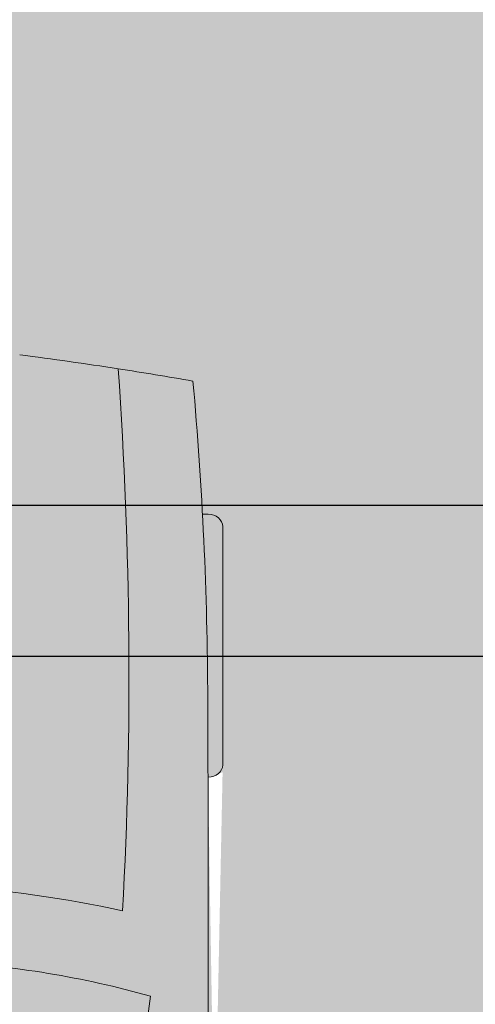
# Model space of a CAD drawing. Units: inches. Extents: x 389 to 971, y 148 to 870.
# Tile 2 of 14: x 529 to 565, y 349 to 428. Entities that reach past the tile are written whole.
import ezdxf

# ---------------------------------------------------------------- set-up
doc = ezdxf.new("R2010")
doc.units = ezdxf.units.IN
doc.header["$MEASUREMENT"] = 0
for name, color, linetype, lineweight in [('A-ANNO-DIMS', 2, 'Continuous', 18), ('C-VEHI', 8, 'Continuous', 13), ('L-GRND-BASE-PATT', 8, 'Continuous', 13)]:
    doc.layers.add(name, color=color, linetype=linetype, lineweight=lineweight)
doc.layers.add('C-VEHI-PATT', color=18, linetype='Continuous', lineweight=13, true_color=0x000000)
doc.layers.add('L-GRND-PATT', color=39, linetype='Continuous', lineweight=13, true_color=0x603913)
doc.styles.get("Standard").update_dxf_attribs({"font": 'arial.ttf'})
doc.dimstyles.get("Standard").update_dxf_attribs({"dimtxt": 8, "dimasz": 8, "dimexe": 0.18, "dimexo": 0.0625, "dimgap": 0.09, "dimtad": 0, "dimtih": 1, "dimtoh": 1, "dimdec": 0, "dimzin": 0, "dimdsep": 46, "dimlunit": 3, "dimtxsty": 'Standard', "dimcen": 0.09, "dimadec": 0, "dimazin": 0, "dimtfac": 1, "dimtdec": 0, "dimtofl": 0, "dimtmove": 0, "dimatfit": 3, "dimfxl": 1, "dimtolj": 1, "dimtzin": 0, "dimarcsym": 0})

# ---------------------------------------------------------------- blocks, each defined once
blk = doc.blocks.new('*U7')
for p, q in [((46.55368679439944, 38.88847654282876), (22.35054758993934, 38.88847654282876)), ((21.10406751471477, 37.40863046792069), (21.10406751471477, 36.83230215753705)), ((47.80016686962392, 37.39011648242055), (47.80016686962392, 37.40863046792069)), ((70.0302824853563, 31.53613089391356), (86.40615155322342, 29.35124891408057))]:
    blk.add_line(p, q)
for centre, major_axis, ratio, start_param, end_param in [((22.35054758993934, 37.40863046792072), (2.08e-14, -1.479846074908118), 0.842303869543976, 3.141592653589776, 4.712388980384677), ((46.55368679439944, 37.40863046792072), (2.2e-14, 1.479846074908118), 0.8423038695439758, -1.570796326794884, 1.73e-14), ((41.19115208863305, -490.8631038926156), (1.294e-13, 528.2339998381949), 0.8423038695439741, 0.0028100083536837, 0.0755983031096952), ((64.48199294511879, -10555.61767587835), (1.907644e-10, 10593.02630634627), 0.842303869543847, -0.0133969486112073, 0.0027970409639888), ((266.0300214172791, -27.52442688366631), (1.966072e-10, 313.3077612809058), 0.8423038695435284, 1.367075990158062, 1.391760499156098), ((135.2911776514449, 5.387441675478555), (2.2715e-12, 81.77258453065997), 0.8423038695439563, 1.245306111696802, 1.507880129813836), ((37.47375371777758, -593.9621830607928), (6.21e-14, -623.32820996736), 0.8423038695439826, 3.09604606856106, 3.200911180495224), ((259.1750197310735, -27.52442688366614), (1.506617e-10, -305.3028914627677), 0.8423038695443789, 4.528606069860317, 4.561837674556238), ((134.4003789125686, 5.387441675477674), (4.276e-13, -89.7774543484738), 0.84230386954398, 4.44948196380473, 4.652344057257214)]:
    blk.add_ellipse(centre, major_axis=major_axis, ratio=ratio, start_param=start_param, end_param=end_param)
blk = doc.blocks.new('*D53')
at = {"layer": 'A-ANNO-DIMS', "color": 0, "lineweight": -2, "transparency": 16777216}
for p, q in [((397.8910240000004, 396.9189020000002), (397.8910240000004, 404.9189020000001)), ((690.1535240000002, 388.9189020000003), (397.7110240000004, 388.9189020000002)), ((690.1535240000002, 376.9189020000001), (397.7110240000005, 376.9189020000001)), ((397.8910240000005, 368.9189020000001), (397.8910240000005, 360.918902))]:
    blk.add_line(p, q, dxfattribs=at)
at = {"layer": 'A-ANNO-DIMS', "color": 0, "transparency": 16777216}
for points in [[(396.5576906666671, 396.9189020000002), (399.2243573333337, 396.9189020000002), (397.8910240000004, 388.9189020000002)], [(396.5576906666671, 368.9189020000001), (399.2243573333338, 368.9189020000001), (397.8910240000005, 376.9189020000001)]]:
    blk.add_solid(points, dxfattribs=at)
at = {"layer": 'Defpoints', "color": 0, "transparency": 16777216}
for p in [(397.8910240000004, 388.9189020000002), (690.2160240000001, 388.9189020000003), (690.2160240000001, 376.9189020000001)]:
    blk.add_point(p, dxfattribs=at)
at = {"layer": 'A-ANNO-DIMS', "color": 0, "transparency": 16777216, "insert": (397.8910240000004, 382.9189019999999), "char_height": 8, "attachment_point": 5}
blk.add_mtext('\\A1;12', dxfattribs=at)

msp = doc.modelspace()

# ---------------------------------------------------------------- hatches: boundary and pattern name
at = {"layer": 'C-VEHI-PATT'}
h = msp.add_hatch(color=256, dxfattribs=at)
h.dxf.hatch_style = 1
edge = h.paths.add_edge_path()
edge.add_ellipse((550.9021553826709, 381.4331108862803), major_axis=(-43.99405423656321, 1.9369e-12), ratio=0.8423038695439613, start_angle=-29.43856959797762, end_angle=1.8189894035458565e-12, ccw=False)
edge.add_line((514.3535105156315, 402.059641051582), (514.3535105156315, 404.7525403567118))
edge.add_ellipse((514.3535105156316, 404.2643898676136), major_axis=(0.5795420236673633, 2e-16), ratio=0.8423038695437671, start_angle=90.00000000001334, end_angle=127.9331304598466)
edge.add_line((514.0354569934393, 404.6724605914631), (509.5535496243029, 402.1940957519602))
edge.add_ellipse((473.3138688667988, 564.9222417143382), major_axis=(196.5636751472093, 8.4793e-12), ratio=0.8423038695439335, start_angle=-80.7434339928015, end_angle=-77.44506735586577, ccw=False)
edge.add_ellipse((535.9119176052684, 201.7546502845751), major_axis=(239.1273775699096, 1.008988e-10), ratio=0.842303869543627, start_angle=100.2095389971183, end_angle=102.4446272934191)
edge.add_ellipse((979.5722266908713, 375.4013592680145), major_axis=(-488.2195497741742, 7.7268e-12), ratio=0.842303869543895, start_angle=-2.863714607837472, end_angle=2.198540565955285)
edge.add_ellipse((510.1338164488812, 299.4839331720496), major_axis=(70.3178640738586, 3.814e-12), ratio=0.8423038695439212, start_angle=94.08241069114638, end_angle=107.71995322274631, ccw=False)
edge.add_line((505.914122382133, 358.6062023341113), (522.79289864913, 358.606202334111))
edge.add_ellipse((518.5732045823792, 299.4839331720493), major_axis=(-70.31786407385354, 1.4408e-12), ratio=0.8423038695439844, start_angle=252.2800467772501, end_angle=265.91758930884987, ccw=False)
edge.add_ellipse((49.13479434038987, 375.4013592680261), major_axis=(-488.2195497741754, 2.5232e-12), ratio=0.8423038695439587, start_angle=177.8014594340444, end_angle=182.8637146078372)
edge.add_ellipse((492.795103425985, 201.7546502845724), major_axis=(239.12737756976, 4.82267e-11), ratio=0.8423038695441539, start_angle=77.5553727065425, end_angle=79.79046100284327)
edge.add_ellipse((555.3931521644682, 564.9222417143374), major_axis=(-196.5636751472384, 3.62381e-11), ratio=0.8423038695438114, start_angle=77.4450673558726, end_angle=80.74343399280832, ccw=False)
edge.add_line((519.1534714069603, 402.19409575196), (514.671564037824, 404.6724605914631))
edge.add_ellipse((514.3535105156316, 404.2643898676136), major_axis=(0.5795420236673633, 2e-16), ratio=0.8423038695437671, start_angle=52.06686954015338, end_angle=90.00000000001334)
edge.add_line((514.3535105156315, 404.7525403567118), (514.3535105156315, 402.0596410515821))
edge.add_ellipse((477.8048656485917, 381.4331108862812), major_axis=(-43.99405423656326, 6.67e-13), ratio=0.8423038695439753, start_angle=180.0000000000002, end_angle=209.4385695979796, ccw=False)
edge.add_line((521.7989198851549, 381.4331108862806), (521.7989198851549, 379.5923831537828))
edge.add_line((521.7989198851549, 379.5923831537828), (523.2258361412675, 379.5923831537828))
edge.add_ellipse((523.0896049791924, 379.1042326646847), major_axis=(0.5795420236669786, 3.601e-13), ratio=0.8423038695443263, start_angle=45.519789117397124, end_angle=89.99999999996442, ccw=False)
edge.add_line((523.4589887688404, 379.4803801228631), (527.8015488731598, 376.4548385069232))
edge.add_line((527.8015488731598, 376.4548385069232), (527.8015488731597, 364.8548231745798))
edge.add_ellipse((524.8002343791572, 364.9712406163019), major_axis=(0.279312372030448, 4.96584264291768), ratio=0.6038335755719146, start_angle=106.34259195429831, end_angle=270.9979857249735, ccw=False)
edge.add_line((521.7989198851548, 364.2715269884119), (521.7989198851549, 381.4331108862806))
edge.add_ellipse((477.8048656485917, 381.4331108862812), major_axis=(-43.99405423656326, 6.67e-13), ratio=0.8423038695439753, start_angle=180.0000000000001, end_angle=209.4385695979795)
edge.add_ellipse((550.9021553826709, 381.4331108862803), major_axis=(-43.99405423656321, 1.9369e-12), ratio=0.8423038695439613, start_angle=-29.43856959797755, end_angle=1.8539e-12)
edge.add_line((506.9081011461076, 381.43311088628), (506.9081011461074, 364.2715269884121))
edge.add_ellipse((503.9067866521049, 364.9712406163021), major_axis=(-0.2793123720310282, 4.965842642917721), ratio=0.6038335755718928, start_angle=89.00201427501901, end_angle=253.6574080456941, ccw=False)
edge.add_line((500.9054721581025, 364.8548231745812), (500.9054721581025, 376.4548385069235))
edge.add_line((500.9054721581025, 376.4548385069235), (505.3530060491612, 379.5535172937331))
edge.add_ellipse((505.61741605207, 379.1042326646849), major_axis=(-0.5795420236672051, 1.236e-13), ratio=0.842303869543997, start_angle=-89.99999999998778, end_angle=-45.51978911742469, ccw=False)
edge.add_line((505.61741605207, 379.5923831537831), (506.9081011461076, 379.5923831537831))
edge.add_line((506.9081011461076, 379.5923831537831), (506.9081011461076, 381.43311088628))
h = msp.add_hatch(color=256, dxfattribs=at)
h.dxf.hatch_style = 1
edge = h.paths.add_edge_path()
edge.add_ellipse((492.795103425985, 201.7546502845724), major_axis=(239.12737756976, 4.82267e-11), ratio=0.8423038695441539, start_angle=77.5553727065425, end_angle=79.79046100284327)
edge.add_ellipse((555.3931521644682, 564.9222417143374), major_axis=(-196.5636751472384, 3.62381e-11), ratio=0.8423038695438114, start_angle=77.4450673558726, end_angle=80.74343399280832, ccw=False)
edge.add_line((519.1534714069603, 402.19409575196), (519.1534714069603, 394.0892586662818))
edge.add_ellipse((477.8048656485917, 381.4331108862812), major_axis=(-43.99405423656326, 6.67e-13), ratio=0.8423038695439753, start_angle=180.0000000000002, end_angle=197.0185128172791, ccw=False)
edge.add_line((521.7989198851549, 381.4331108862806), (521.7989198851549, 379.5923831537828))
edge.add_line((521.7989198851549, 379.5923831537828), (523.1794038652976, 379.5923831537828))
edge.add_ellipse((523.0896049791924, 379.1042326646847), major_axis=(0.5795420236669786, 3.601e-13), ratio=0.8423038695443263, start_angle=45.519789117397124, end_angle=89.99999999996442, ccw=False)
edge.add_line((523.4589887688405, 379.480380122863), (527.8015488731598, 376.4548385069232))
edge.add_line((527.8015488731598, 376.4548385069232), (527.8015488731597, 364.8548231745798))
edge.add_ellipse((524.8002343791572, 364.9712406163019), major_axis=(0.279312372030448, 4.96584264291768), ratio=0.6038335755719146, start_angle=106.34259195429831, end_angle=270.9979857249735, ccw=False)
edge.add_line((521.7989198851548, 364.2715269884119), (521.7989198851549, 381.4331108862806))
edge.add_ellipse((477.8048656485917, 381.4331108862812), major_axis=(-43.99405423656326, 6.67e-13), ratio=0.8423038695439753, start_angle=180.0000000000001, end_angle=197.018512817279)
edge.add_line((519.1534714069603, 394.0892586662818), (519.1534714069603, 358.6062023341111))
edge.add_line((519.1534714069603, 358.6062023341111), (522.79289864913, 358.606202334111))
edge.add_ellipse((518.5732045823792, 299.4839331720493), major_axis=(-70.31786407385354, 1.4408e-12), ratio=0.8423038695439844, start_angle=252.2800467772501, end_angle=265.91758930884987, ccw=False)
edge.add_ellipse((49.13479434038987, 375.4013592680261), major_axis=(-488.2195497741754, 2.5232e-12), ratio=0.8423038695439587, start_angle=177.8014594340444, end_angle=182.8637146078372)
h = msp.add_hatch(color=256, dxfattribs=at)
h.dxf.hatch_style = 1
edge = h.paths.add_edge_path(flags=16)
edge.add_ellipse((3386.011413077446, 329.726312794031), major_axis=(-2896.629999631248, 1.069454e-10), ratio=0.8423038695494893, start_angle=-0.1208973690315247, end_angle=0.3640763488915013, ccw=False)
edge.add_line((489.3905023836935, 335.8383575186984), (486.2179253655185, 346.1978202249628))
edge.add_ellipse((8782.002602781096, 354.247254279773), major_axis=(-8295.790181758603, 9.87839e-10), ratio=0.8423038695486498, start_angle=0.0555943135052214, end_angle=0.3777641939157137)
edge.add_line((486.4665645878948, 299.5520931219791), (489.4638383140943, 311.3204429697198))
edge = h.paths.add_edge_path(flags=16)
edge.add_ellipse((512.1608573463288, 287.5825181681774), major_axis=(62.33048198263887, 2.0798e-12), ratio=0.8423038695439498, start_angle=94.8700695971331, end_angle=112.791914877584)
edge.add_line((491.3642517254777, 337.0752369161335), (489.6529508739416, 349.9015767089268))
edge.add_ellipse((510.1338164488795, 298.7862183048575), major_axis=(64.04807894948699, 3.9006e-12), ratio=0.8423038695439252, start_angle=94.27742096304979, end_angle=111.83495379670401, ccw=False)
edge.add_line((506.1068129054811, 352.6274231954524), (522.600208125781, 352.6274231954521))
edge.add_ellipse((518.5732045823798, 298.7862183048586), major_axis=(64.04807894948067, 3.24e-14), ratio=0.8423038695439885, start_angle=68.16504620328948, end_angle=85.72257903694378, ccw=False)
edge.add_line((539.05407015732, 349.9015767089259), (537.3427693057835, 337.0752369161327))
edge.add_ellipse((516.5461636849332, 287.5825181681899), major_axis=(62.33048198262021, 1.5954e-12), ratio=0.8423038695439995, start_angle=67.20808512240782, end_angle=85.12993040286212)
edge.add_line((521.0080028322477, 339.9490379899644), (507.6990181990146, 339.9490379899646))
edge = h.paths.add_edge_path(flags=16)
edge.add_ellipse((514.3535105156315, 391.3730654902235), major_axis=(-115.1512533244504, 1.8736e-12), ratio=0.8423038695439684, start_angle=76.4018653097696, end_angle=103.5981346902308)
edge.add_line((537.3427693057832, 296.3333211885938), (537.342769305783, 281.5897392316151))
edge.add_ellipse((514.3535105156313, 376.6294835332447), major_axis=(-115.1512533244486, 9.02e-13), ratio=0.8423038695439828, start_angle=76.40186530976922, end_angle=103.59813469023032, ccw=False)
edge.add_line((491.3642517254773, 281.5897392316156), (491.3642517254774, 296.3333211885945))
edge = h.paths.add_edge_path()
edge.add_ellipse((8782.002602781105, 354.2472542798386), major_axis=(-8296.949265805946, 5.39345e-11), ratio=0.8423038695428886, start_angle=0.3838667787920247, end_angle=0.5282714718170651)
edge.add_ellipse((8782.002602781105, 354.2472542798386), major_axis=(-8296.949265805946, 5.39345e-11), ratio=0.8423038695428886, start_angle=0.5282714718170651, end_angle=0.6465540970606384)
edge.add_ellipse((488.1158467995968, 260.6509346628684), major_axis=(2.318168094668909, 7.48e-14), ratio=0.8423038695439647, start_angle=180.6465540970884, end_angle=269.9999999999081)
edge.add_line((488.115846799593, 258.6983327064755), (491.3642517254771, 258.6983327064753))
edge.add_line((491.3642517254771, 258.6983327064753), (491.3642517254771, 274.201106836649))
edge.add_ellipse((493.6824198201462, 273.9438556676354), major_axis=(-2.318168094668919, 1.896e-13), ratio=0.8423038695439611, start_angle=-89.99999999999523, end_angle=4.718003765447065e-12, ccw=False)
edge.add_line((493.6824198201462, 275.8964576240284), (535.3300149439905, 275.8964576240277))
edge.add_ellipse((535.024601211114, 273.9438556676347), major_axis=(2.318168094668976, 2.946e-13), ratio=0.8423038695439647, start_angle=-7.275957614183426e-12, end_angle=89.99999999998943, ccw=False)
edge.add_line((537.342769305783, 273.9438556676347), (537.3427693057827, 258.698332706474))
edge.add_line((537.3427693057827, 258.698332706474), (540.591174231666, 258.6983327064739))
edge.add_ellipse((540.5911742316634, 260.6509346628669), major_axis=(-2.318168094668839, 2.143e-13), ratio=0.8423038695440144, start_angle=90.00000000008203, end_angle=179.3534459029346)
edge.add_ellipse((-7753.295581726658, 354.2472542799028), major_axis=(-8296.949265782761, 2.068448e-10), ratio=0.8423038695442414, start_angle=179.3534459029388, end_angle=179.3813568036815)
edge.add_ellipse((-7753.295581726658, 354.2472542799028), major_axis=(-8296.949265782761, 2.068448e-10), ratio=0.8423038695442414, start_angle=179.3813568036815, end_angle=179.4717285281828)
edge.add_ellipse((-7753.295581726658, 354.2472542799028), major_axis=(-8296.949265782761, 2.068448e-10), ratio=0.8423038695442414, start_angle=179.4717285281828, end_angle=179.6161332212082)
edge.add_ellipse((-7753.295581726658, 354.2472542799028), major_axis=(-8296.949265782761, 2.068448e-10), ratio=0.8423038695442414, start_angle=179.6161332212082, end_angle=180.090229088595)
edge.add_ellipse((-7753.295581726658, 354.2472542799028), major_axis=(-8296.949265782761, 2.068448e-10), ratio=0.8423038695442414, start_angle=180.090229088595, end_angle=180.134986576859)
edge.add_ellipse((129.8867725257751, 372.4897205359271), major_axis=(-413.7373561031673, 2.44623e-11), ratio=0.8423038695441432, start_angle=180.1806905311865, end_angle=182.1799503136479)
edge.add_ellipse((129.8867725257751, 372.4897205359271), major_axis=(-413.7373561031673, 2.44623e-11), ratio=0.8423038695441432, start_angle=182.1799503136479, end_angle=183.6504275857017)
edge.add_ellipse((492.7951034259847, 196.3854951855023), major_axis=(245.3971626940514, 1.422861e-10), ratio=0.8423038695444116, start_angle=76.21947101046817, end_angle=77.87403444768196)
edge.add_ellipse((49.13479434038987, 375.4013592680261), major_axis=(-488.2195497741754, 2.5232e-12), ratio=0.8423038695439587, start_angle=177.8014594340445, end_angle=182.8637146078372, ccw=False)
edge.add_ellipse((518.5732045823792, 299.4839331720493), major_axis=(-70.31786407385354, 1.4408e-12), ratio=0.8423038695439844, start_angle=252.2800467772501, end_angle=265.9175893088498)
edge.add_line((522.79289864913, 358.606202334111), (505.9141223821329, 358.6062023341113))
edge.add_ellipse((510.1338164488812, 299.4839331720496), major_axis=(70.3178640738586, 3.814e-12), ratio=0.8423038695439212, start_angle=94.08241069114636, end_angle=107.7199532227462)
edge.add_ellipse((979.5722266908713, 375.4013592680145), major_axis=(-488.2195497741742, 7.7268e-12), ratio=0.842303869543895, start_angle=-2.863714607837494, end_angle=2.198540565955284, ccw=False)
edge.add_ellipse((535.9119176052733, 196.3854951855018), major_axis=(-245.3971626940985, 1.013648e-10), ratio=0.8423038695442548, start_angle=-77.87403444769295, end_angle=-76.2194710104792)
edge.add_ellipse((898.8202485054873, 372.489720535918), major_axis=(413.7373561031672, 1.26113e-11), ratio=0.8423038695441164, start_angle=176.3495724142985, end_angle=177.8200496863523)
edge.add_ellipse((898.8202485054873, 372.489720535918), major_axis=(413.7373561031672, 1.26113e-11), ratio=0.8423038695441164, start_angle=177.8200496863523, end_angle=179.8643876095591)
edge.add_ellipse((8782.002602781105, 354.2472542798386), major_axis=(-8296.949265805946, 5.39345e-11), ratio=0.8423038695428886, start_angle=-0.1349865768573029, end_angle=-0.090229088593484)
edge.add_ellipse((8782.002602781105, 354.2472542798386), major_axis=(-8296.949265805946, 5.39345e-11), ratio=0.8423038695428886, start_angle=-0.090229088593484, end_angle=0.3838667787920247)
edge = h.paths.add_edge_path(flags=16)
edge.add_ellipse((-2357.304392046186, 329.7263127941099), major_axis=(2896.629999631251, 5.35614e-11), ratio=0.8423038695445265, start_angle=-0.3640763488920631, end_angle=0.1208973690309369)
edge.add_line((539.3165186475693, 335.8383575187012), (542.4890956657468, 346.1978202249727))
edge.add_ellipse((-7753.295581749842, 354.2472542800017), major_axis=(8295.790181758617, 3.2664368e-09), ratio=0.8423038695525207, start_angle=-0.37776419393310334, end_angle=-0.055594313522590255, ccw=False)
edge.add_line((542.240456443367, 299.5520931219743), (539.2431827171666, 311.3204429697195))
h = msp.add_hatch(color=256, dxfattribs=at)
h.dxf.hatch_style = 1
edge = h.paths.add_edge_path()
edge.add_ellipse((543.6536840561057, 387.2465553762822), major_axis=(-1.159084047334545, 1.527e-13), ratio=0.8423038695438989, start_angle=180.0000000000075, end_angle=270.0000000000075)
edge.add_line((543.6536840561057, 388.2228563544787), (543.2022770064673, 388.2228563544788))
edge.add_ellipse((129.8867725257751, 372.4897205359271), major_axis=(-413.7373561031673, 2.44623e-11), ratio=0.8423038695441432, start_angle=180.1806905311866, end_angle=182.179950313648, ccw=False)
edge.add_ellipse((129.8867725257751, 372.4897205359271), major_axis=(-413.7373561031673, 2.44623e-11), ratio=0.8423038695441432, start_angle=180.1356123904411, end_angle=180.1806905311866, ccw=False)
edge.add_ellipse((-7753.295581726658, 354.2472542799028), major_axis=(-8296.949265782761, 2.068448e-10), ratio=0.8423038695442414, start_angle=180.0902290885951, end_angle=180.1349865768591, ccw=False)
edge.add_line((543.6391830444066, 367.3132337842714), (543.6536840561062, 367.3132337842714))
edge.add_ellipse((543.6536840561054, 368.2895347624679), major_axis=(1.159084047334544, 7.24e-14), ratio=0.8423038695439478, start_angle=269.9999999999964, end_angle=359.9999999999964)
edge.add_line((544.8127681034399, 368.2895347624669), (544.8127681034401, 387.2465553762833))
h = msp.add_hatch(color=256, dxfattribs=at)
h.dxf.hatch_style = 1
edge = h.paths.add_edge_path()
edge.add_ellipse((518.5732045823798, 298.7862183048586), major_axis=(64.04807894948067, 3.24e-14), ratio=0.8423038695439885, start_angle=68.16504620328955, end_angle=85.72257903694374)
edge.add_line((522.600208125781, 352.6274231954521), (506.106812905481, 352.6274231954524))
edge.add_ellipse((510.1338164488795, 298.7862183048575), major_axis=(64.04807894948699, 3.9006e-12), ratio=0.8423038695439252, start_angle=94.2774209630498, end_angle=111.834953796704)
edge.add_line((489.6529508739416, 349.9015767089268), (491.3642517254777, 337.0752369161335))
edge.add_ellipse((512.1608573463288, 287.5825181681774), major_axis=(62.33048198263887, 2.0798e-12), ratio=0.8423038695439498, start_angle=94.87006959713312, end_angle=112.79191487758399, ccw=False)
edge.add_line((507.6990181990146, 339.9490379899646), (521.0080028322477, 339.9490379899644))
edge.add_ellipse((516.5461636849332, 287.5825181681899), major_axis=(62.33048198262021, 1.5954e-12), ratio=0.8423038695439995, start_angle=67.2080851224078, end_angle=85.1299304028621, ccw=False)
edge.add_line((537.3427693057835, 337.0752369161327), (539.05407015732, 349.9015767089259))
at = {"layer": 'L-GRND-BASE-PATT'}
h = msp.add_hatch(color=256, dxfattribs=at)
h.dxf.hatch_style = 1
edge = h.paths.add_edge_path(flags=16)
edge.add_ellipse((8782.002602781105, 354.2472542798386), major_axis=(-8296.949265805946, 5.39345e-11), ratio=0.8423038695428886, start_angle=-0.0902290885933894, end_angle=0.3838667787920258, ccw=False)
edge.add_ellipse((485.0533369751568, 368.2895347624687), major_axis=(-1.159084047334488, 1.838e-13), ratio=0.8423038695439892, start_angle=9.094947017729282e-12, end_angle=90.00000000000898, ccw=False)
edge.add_line((483.8942529278224, 368.2895347624687), (483.8942529278225, 387.6039063360424))
edge.add_ellipse((485.0533369751571, 387.2465553762829), major_axis=(1.159084047334488, 1.838e-13), ratio=0.8423038695439892, start_angle=89.99999999999102, end_angle=179.9999999999909, ccw=False)
edge.add_line((485.0533369751572, 388.2228563544795), (485.5047440247956, 388.2228563544795))
edge.add_ellipse((898.8202485054873, 372.489720535918), major_axis=(413.7373561031672, 1.26113e-11), ratio=0.8423038695441164, start_angle=176.3495724142986, end_angle=177.8200496863524, ccw=False)
edge.add_ellipse((535.9119176052733, 196.3854951855018), major_axis=(-245.3971626940985, 1.013648e-10), ratio=0.8423038695442548, start_angle=-77.87403444769302, end_angle=-76.2194710104792, ccw=False)
edge.add_ellipse((535.9119176052684, 201.7546502845751), major_axis=(239.1273775699096, 1.008988e-10), ratio=0.842303869543627, start_angle=100.20953899711827, end_angle=102.44462729341922, ccw=False)
edge.add_ellipse((473.3138688667988, 564.9222417143382), major_axis=(196.5636751472093, 8.4793e-12), ratio=0.8423038695439335, start_angle=-80.74343399280163, end_angle=-77.44506735586587)
edge.add_line((509.5535496243029, 402.1940957519602), (514.3535105156315, 404.8483349684994))
edge.add_line((514.3535105156315, 404.8483349684994), (514.3535105156315, 404.7971763262221))
edge.add_ellipse((514.3535105156316, 404.2643898676136), major_axis=(0.5795420236673633, 2e-16), ratio=0.8423038695437671, start_angle=52.06686954015339, end_angle=90.00000000001342, ccw=False)
edge.add_line((514.671564037824, 404.672460591463), (519.1534714069603, 402.19409575196))
edge.add_ellipse((555.3931521644682, 564.9222417143374), major_axis=(-196.5636751472384, 3.62381e-11), ratio=0.8423038695438114, start_angle=77.44506735587258, end_angle=80.74343399280833)
edge.add_ellipse((492.795103425985, 201.7546502845724), major_axis=(239.12737756976, 4.82267e-11), ratio=0.8423038695441539, start_angle=77.55537270654253, end_angle=79.7904610028433, ccw=False)
edge.add_ellipse((492.7951034259847, 196.3854951855023), major_axis=(245.3971626940514, 1.422861e-10), ratio=0.8423038695444116, start_angle=76.21947101046823, end_angle=77.87403444768199, ccw=False)
edge.add_ellipse((129.8867725257751, 372.4897205359271), major_axis=(-413.7373561031673, 2.44623e-11), ratio=0.8423038695441432, start_angle=182.179950313648, end_angle=183.6504275857018, ccw=False)
edge.add_line((543.2022770064673, 388.2228563544788), (544.0779382625514, 388.2228563544787))
edge.add_ellipse((543.6536840561057, 387.2465553762822), major_axis=(-1.159084047334545, 1.527e-13), ratio=0.8423038695438989, start_angle=180.0000000000075, end_angle=270.00000000000756, ccw=False)
edge.add_line((544.8127681034401, 387.2465553762826), (544.8127681034399, 367.9321838027083))
edge.add_ellipse((543.6536840561054, 368.2895347624679), major_axis=(1.159084047334544, 7.24e-14), ratio=0.8423038695439478, start_angle=269.9999999999964, end_angle=359.9999999999964, ccw=False)
edge.add_ellipse((-7753.295581726658, 354.2472542799028), major_axis=(-8296.949265782761, 2.068448e-10), ratio=0.8423038695442414, start_angle=179.6161332212083, end_angle=180.0902290885951, ccw=False)
edge.add_line((543.3912265319653, 298.6607849184036), (544.0779382625504, 298.6607849184036))
edge.add_ellipse((543.6536840561046, 297.6844839402071), major_axis=(1.159084047334431, 1.769e-13), ratio=0.8423038695439814, start_angle=-1.1482370609883219e-11, end_angle=89.99999999999119, ccw=False)
edge.add_line((544.8127681034391, 297.684483940207), (544.8127681034387, 278.3701123666333))
edge.add_ellipse((543.6536840561043, 278.727463326393), major_axis=(-1.159084047334431, 2.574e-13), ratio=0.8423038695440306, start_angle=90.00000000001268, end_angle=180.0000000000099, ccw=False)
edge.add_line((543.6536840561045, 277.7511623481965), (543.1566278692261, 277.7511623481965))
edge.add_ellipse((-7753.295581726658, 354.2472542799028), major_axis=(-8296.949265782761, 2.068448e-10), ratio=0.8423038695442414, start_angle=179.3813568036816, end_angle=179.4717285281829, ccw=False)
edge.add_ellipse((542.4236240941387, 263.2762864208561), major_axis=(-1.738626071001761, 2.132e-13), ratio=0.8423038695439151, start_angle=179.3717627838137, end_angle=248.464756601011, ccw=False)
edge.add_ellipse((-7753.875123750511, 354.2472542780016), major_axis=(-8298.740341433751, 2.4782644722e-06), ratio=0.8423038662721074, start_angle=179.3534459200609, end_angle=179.3717628008941, ccw=False)
edge.add_ellipse((540.0116322079951, 260.6509346628677), major_axis=(-4.109243751168186, 2.384e-13), ratio=0.842303869543976, start_angle=90.0000000000635, end_angle=179.3534459029233, ccw=False)
edge.add_line((540.0116322079991, 257.1897027503593), (488.6953888232593, 257.1897027503609))
edge.add_ellipse((488.6953888232669, 260.6509346628715), major_axis=(4.10924375117072, 1.262e-13), ratio=0.8423038695439824, start_angle=180.6465540970565, end_angle=269.9999999998589, ccw=False)
edge.add_ellipse((8782.582144816053, 354.2472542821698), major_axis=(-8298.740341477976, 1.8591886369e-06), ratio=0.8423038720186145, start_angle=0.6282372290784792, end_angle=0.6465541099116194, ccw=False)
edge.add_ellipse((486.2833969371199, 263.2762864208594), major_axis=(-1.738626071002378, 2.7e-13), ratio=0.8423038695439394, start_angle=-68.46475649596817, end_angle=0.6282372161796275, ccw=False)
edge.add_ellipse((8782.002602781105, 354.2472542798386), major_axis=(-8296.949265805946, 5.39345e-11), ratio=0.8423038695428886, start_angle=0.5282714718171064, end_angle=0.6465540970606867, ccw=False)
edge.add_line((485.5503931620382, 277.7511623481972), (484.6290827687102, 277.7511623481972))
edge.add_ellipse((485.0533369751559, 278.7274633263938), major_axis=(-1.159084047334545, 3.11e-13), ratio=0.8423038695439968, start_angle=1.5404566511278972e-11, end_angle=90.000000000012, ccw=False)
edge.add_line((483.8942529278214, 278.7274633263938), (483.8942529278216, 298.0418348999672))
edge.add_ellipse((485.053336975156, 297.6844839402078), major_axis=(1.159084047334488, 1.025e-13), ratio=0.8423038695440382, start_angle=89.99999999999488, end_angle=179.9999999999949, ccw=False)
edge = h.paths.add_edge_path(flags=0)
edge.add_ellipse((8782.002602781096, 354.247254279773), major_axis=(-8295.790181758603, 9.87839e-10), ratio=0.8423038695486498, start_angle=0.05559431350519617, end_angle=0.37776419391582294, ccw=False)
edge.add_line((486.2179253655185, 346.1978202249628), (489.3905023836935, 335.8383575186984))
edge.add_ellipse((3386.011413077446, 329.726312794031), major_axis=(-2896.629999631248, 1.069454e-10), ratio=0.8423038695494893, start_angle=-0.1208973690315206, end_angle=0.3640763488915184)
edge.add_line((489.4638383140943, 311.3204429697198), (486.4665645878948, 299.5520931219791))
edge = h.paths.add_edge_path(flags=0)
edge.add_ellipse((514.3535105156315, 391.3730654902235), major_axis=(-115.1512533244504, 1.8736e-12), ratio=0.8423038695439684, start_angle=76.4018653097696, end_angle=103.5981346902308)
edge.add_line((537.3427693057832, 296.3333211885938), (537.342769305783, 281.5897392316151))
edge.add_ellipse((514.3535105156313, 376.6294835332447), major_axis=(-115.1512533244486, 9.02e-13), ratio=0.8423038695439828, start_angle=76.40186530976922, end_angle=103.59813469023032, ccw=False)
edge.add_line((491.3642517254773, 281.5897392316156), (491.3642517254774, 296.3333211885945))
edge = h.paths.add_edge_path(flags=0)
edge.add_line((491.3642517254777, 337.0752369161334), (489.6529508739416, 349.9015767089268))
edge.add_ellipse((510.1338164488795, 298.7862183048575), major_axis=(64.04807894948699, 3.9006e-12), ratio=0.8423038695439252, start_angle=94.27742096304979, end_angle=111.83495379670401, ccw=False)
edge.add_line((506.106812905481, 352.6274231954524), (522.600208125781, 352.6274231954521))
edge.add_ellipse((518.5732045823798, 298.7862183048586), major_axis=(64.04807894948067, 3.24e-14), ratio=0.8423038695439885, start_angle=68.16504620328948, end_angle=85.72257903694378, ccw=False)
edge.add_line((539.05407015732, 349.9015767089259), (537.3427693057835, 337.0752369161327))
edge.add_ellipse((516.5461636849332, 287.5825181681899), major_axis=(62.33048198262021, 1.5954e-12), ratio=0.8423038695439995, start_angle=67.20808512240782, end_angle=85.12993040286212)
edge.add_line((521.0080028322477, 339.9490379899644), (507.6990181990146, 339.9490379899646))
edge.add_ellipse((512.1608573463288, 287.5825181681774), major_axis=(62.33048198263887, 2.0798e-12), ratio=0.8423038695439498, start_angle=94.8700695971331, end_angle=112.791914877584)
edge = h.paths.add_edge_path(flags=0)
edge.add_ellipse((493.6824198201462, 273.9438556676354), major_axis=(-2.318168094668919, 1.896e-13), ratio=0.8423038695439611, start_angle=-89.99999999999523, end_angle=4.718003765447065e-12, ccw=False)
edge.add_line((493.6824198201462, 275.8964576240284), (535.3743409680425, 275.8964576240277))
edge.add_ellipse((535.024601211114, 273.9438556676347), major_axis=(2.318168094668976, 2.946e-13), ratio=0.8423038695439647, start_angle=-7.275957614183426e-12, end_angle=89.99999999998943, ccw=False)
edge.add_line((537.342769305783, 273.9438556676347), (537.3427693057827, 258.698332706474))
edge.add_line((537.3427693057827, 258.698332706474), (540.5911742316662, 258.6983327064739))
edge.add_ellipse((540.5911742316634, 260.6509346628669), major_axis=(-2.318168094668839, 2.143e-13), ratio=0.8423038695440144, start_angle=90.00000000008203, end_angle=179.3534459029346)
edge.add_line((540.5911742316662, 258.6983327064739), (487.7691399811528, 258.6983327064755))
edge.add_ellipse((488.1158467995968, 260.6509346628684), major_axis=(2.318168094668909, 7.48e-14), ratio=0.8423038695439647, start_angle=180.6465540970884, end_angle=269.9999999999081)
edge.add_line((488.1158467995931, 258.6983327064755), (491.3642517254771, 258.6983327064754))
edge.add_line((491.3642517254771, 258.6983327064754), (491.3642517254771, 274.2384428182294))
h.paths.add_polyline_path([(746.1375687288224, 327.3223047166553), (750.1400147212453, 327.3223047166553), (750.1400147212453, 326.2830696147227), (798.1693712998389, 326.2830696147227), (798.1693712998389, 327.3223047166553), (802.1718172922616, 327.3223047166553), (802.1718172922616, 309.9783792024682, -0.1904762075443491), (746.1375687288224, 309.9783668090107)], flags=16)
h.paths.add_polyline_path([(782.1595875801748, 313.5684994305933), (782.1595893317732, 309.0414930416419, -0.0496282101666581), (766.1497986905329, 309.0414910503953), (766.1498004421323, 313.5684994305933)], flags=0)
h.paths.add_polyline_path([(755.1858908233534, 344.9352232902417), (755.1858908233534, 373.916311072083), (788.1243995226009, 373.916311072083), (788.1243995226009, 344.9352232902417)], flags=16)
h.paths.add_polyline_path([(757.1858908233535, 346.9352232902417), (757.1858908233535, 371.916311072083), (786.1243995226009, 371.916311072083), (786.1243995226009, 346.9352232902417)], flags=0)
h.paths.add_polyline_path([(803.6445810111745, 338.4878931208803), (803.6445810111745, 342.4903391133031), (804.6838161131072, 342.4903391133031), (804.6838161131072, 390.5196956918968), (803.6445810111748, 390.5196956918968), (803.6445810111748, 394.5221416843196), (820.9885065253617, 394.5221416843196, -0.1904762075443491), (820.9885189188192, 338.4878931208803)], flags=16)
h.paths.add_polyline_path([(806.8706930931005, 326.6963103558256), (806.4254411777042, 327.1415622712219), (806.4723791864895, 326.6297175483474)], flags=16)
h.paths.add_polyline_path([(822.0328146004263, 317.4007976138144), (822.1941503181826, 317.8932883068639), (821.562628166435, 317.9885306563034)], flags=16)
h.paths.add_polyline_path([(817.3983862972365, 358.5001248341902), (817.3983862972365, 374.5099119722327), (821.9253926861879, 374.5099137238312, -0.049628210166658), (821.9253946774346, 358.5001230825909)], flags=0)
h.paths.add_polyline_path([(808.1446344648577, 418.9736619306146), (808.2246858861593, 418.5632188717996), (808.5395491501399, 418.5787472453325)], flags=16)
h.paths.add_polyline_path([(820.3158762739024, 412.6690288868844), (820.4772119916585, 413.161519579934), (819.8456898399113, 413.2567619293735)], flags=16)
h.paths.add_polyline_path([(466.3155093563569, 235.5246322146605), (517.3806533266912, 235.5246322146605), (517.3806533266912, 244.4269231682286), (466.3155093563569, 244.4269231682286)], flags=24)
h.paths.add_polyline_path([(739.8737195480014, 256.2000079819968), (815.4040239338423, 256.2000079819968), (815.4040239338423, 265.3453807094367), (739.8737195480014, 265.3453807094367)], flags=24)
h.paths.add_polyline_path([(750.6081538187397, 393.6666679930368), (791.5680640722773, 393.6666679930368), (791.5680640722773, 412.3933175868746), (750.6081538187397, 412.3933175868746)], flags=24)
h.paths.add_polyline_path([(438.9630812812552, 410.0618566955462), (484.6203810968238, 410.0618566955462), (484.6203810968238, 429.1217352891893), (438.9630812812552, 429.1217352891893)], flags=24)
edge = h.paths.add_edge_path()
edge.add_line((839.2160244416713, 285.6445131961097), (611.8786784019748, 285.6445131961099))
edge.add_line((611.8786784019748, 285.6445131961099), (604.3870116090119, 285.6445131961097))
edge.add_line((604.3870116090119, 285.6445131961097), (595.3870116090119, 285.6445131961097))
edge.add_line((595.3870116090119, 285.6445131961097), (595.3870116090118, 370.1553848722774))
edge.add_line((595.3870116090118, 370.1553848722774), (604.0816928471932, 370.1553848722774))
edge.add_line((604.0816928471932, 370.1553848722774), (604.0816928471932, 371.3788335667469))
edge.add_line((604.0816928471932, 371.3788335667469), (632.0194586761203, 371.3788335667469))
edge.add_arc((604.0816928471932, 370.1553848722773), 27.96454158787471, 2.507490703587644, 90.00000000000003)
edge.add_line((604.0816928471932, 398.1199264601519), (599.8870116090108, 398.1652144688576))
edge.add_line((599.8870116090108, 398.1652144688576), (604.4225424425357, 398.1652144688576))
edge.add_arc((604.4225424425357, 428.4020866923496), 30.23687222349201, 270.0000000000002, 357.492509296413)
edge.add_line((634.6304631740308, 427.0792235325719), (604.4225424425357, 427.0792235325719))
edge.add_line((604.4225424425357, 427.0792235325719), (604.4225424425357, 428.4020866923497))
edge.add_line((604.4225424425357, 428.4020866923497), (599.8870116090119, 428.4020866923497))
edge.add_line((599.8870116090119, 428.4020866923497), (595.3870116090116, 428.4020866923497))
edge.add_line((595.3870116090116, 428.4020866923497), (595.3870116090118, 434.6445131961097))
edge.add_line((595.3870116090118, 434.6445131961097), (585.0790669792458, 434.6445131961097))
edge.add_line((585.0790669792458, 434.6445131961097), (540.3921730610418, 434.6445131961097))
edge.add_line((540.3921730610418, 434.6445131961097), (526.712508448134, 434.6445131961097))
edge.add_line((526.712508448134, 434.6445131961097), (488.4094553949635, 434.6445131961097))
edge.add_line((488.4094553949635, 434.6445131961097), (432.2160244416713, 434.6445131961097))
edge.add_line((432.2160244416713, 434.6445131961097), (432.2160244416713, 243.6445131961098))
edge.add_line((432.2160244416713, 243.6445131961098), (437.2160244416714, 243.6445131961098))
edge.add_line((437.2160244416714, 243.6445131961098), (437.2160244416714, 234.6445131961098))
edge.add_line((437.2160244416714, 234.6445131961098), (581.2160244416713, 234.6445131961098))
edge.add_line((581.2160244416713, 234.6445131961098), (581.2160244416713, 238.6445131961097))
edge.add_line((581.2160244416713, 238.6445131961097), (581.2160244416713, 243.6445131961098))
edge.add_line((581.2160244416713, 243.6445131961098), (590.2160244416713, 243.6445131961098))
edge.add_line((590.2160244416713, 243.6445131961098), (590.2160244416713, 238.6445131961097))
edge.add_line((590.2160244416713, 238.6445131961097), (839.2160244416713, 238.6445131961098))
edge.add_line((839.2160244416713, 238.6445131961098), (839.2160244416713, 285.6445131961097))
at = {"layer": 'L-GRND-PATT'}
h = msp.add_hatch(dxfattribs=at)
h.set_pattern_fill('EARTH', color=256, angle=45)
h.set_pattern_definition([(45, (0, 0), (0, 8.980256121069154), [6.349999999999999, -6.349999999999999]), (45, (-1.683798022700466, 1.683798022700466), (0, 8.980256121069154), [6.349999999999999, -6.349999999999999]), (45, (-3.367596045400933, 3.367596045400933), (0, 8.980256121069154), [6.349999999999999, -6.349999999999999]), (135, (-3.367596045400933, 4.490128060534576), (-8.980256121069154, 0), [6.349999999999999, -6.349999999999999]), (135, (-1.683798022700466, 6.173926083235043), (-8.980256121069154, 0), [6.349999999999999, -6.349999999999999]), (135, (0, 7.85772410593551), (-8.980256121069154, 0), [6.349999999999999, -6.349999999999999])])
h.paths.add_polyline_path([(432.2160244416713, 243.6445131961098), (437.2160244416714, 243.6445131961098), (437.2160244416714, 234.6445131961098), (581.2160244416713, 234.6445131961098), (581.2160244416713, 238.6445131961097), (581.2160244416713, 243.6445131961098), (590.2160244416713, 243.6445131961098), (590.2160244416713, 238.6445131961097), (839.2160244416713, 238.6445131961098), (839.2160244416712, 285.6445131961097), (810.0513609197296, 285.6445131961097), (733.8056934525983, 285.6445131961099), (684.2433676403508, 285.6445131961098), (611.8786784019748, 285.6445131961099), (604.3870116090119, 285.6445131961097), (595.3870116090119, 285.6445131961097), (595.3870116090118, 370.1553848722774), (604.0816928471932, 370.1553848722774), (604.0816928471932, 371.3788335667469), (632.0194586761203, 371.3788335667469, 0.4014527144963568), (604.0816928471932, 398.119926460152), (599.8870116090127, 398.1652144688576), (604.4225424425357, 398.1652144688576, 0.4014527144963579), (634.6304631740308, 427.0792235325719), (604.4225424425357, 427.0792235325719), (604.4225424425357, 428.4020866923497), (599.8870116090119, 428.4020866923497), (595.3870116090116, 428.4020866923497), (595.3870116090118, 434.6445131961097), (585.0790669792458, 434.6445131961097), (540.3921730610418, 434.6445131961097), (526.712508448134, 434.6445131961097), (488.4094553949635, 434.6445131961097), (432.2160244416713, 434.6445131961097)])
edge = h.paths.add_edge_path(flags=16)
edge.add_line((483.8942529278214, 278.7274633263938), (483.8942529278216, 298.2563878122772))
edge.add_ellipse((485.053336975156, 297.6844839402078), major_axis=(1.159084047334488, 1.025e-13), ratio=0.8423038695440382, start_angle=89.99999999999488, end_angle=179.9999999999949, ccw=False)
edge.add_ellipse((8782.002602781105, 354.2472542798386), major_axis=(-8296.949265805946, 5.39345e-11), ratio=0.8423038695428886, start_angle=-0.0902290885933894, end_angle=0.3838667787920258, ccw=False)
edge.add_ellipse((485.0533369751568, 368.2895347624687), major_axis=(-1.159084047334488, 1.838e-13), ratio=0.8423038695439892, start_angle=9.094947017729282e-12, end_angle=90.00000000000898, ccw=False)
edge.add_line((483.8942529278224, 368.2895347624687), (483.8942529278225, 387.8184592483523))
edge.add_ellipse((485.0533369751571, 387.2465553762829), major_axis=(1.159084047334488, 1.838e-13), ratio=0.8423038695439892, start_angle=89.99999999999102, end_angle=179.9999999999909, ccw=False)
edge.add_ellipse((898.8202485054873, 372.489720535918), major_axis=(413.7373561031672, 1.26113e-11), ratio=0.8423038695441164, start_angle=176.3495724142986, end_angle=177.8200496863524, ccw=False)
edge.add_ellipse((535.9119176052733, 196.3854951855018), major_axis=(-245.3971626940985, 1.013648e-10), ratio=0.8423038695442548, start_angle=-77.87403444769302, end_angle=-76.2194710104792, ccw=False)
edge.add_ellipse((535.9119176052684, 201.7546502845751), major_axis=(239.1273775699096, 1.008988e-10), ratio=0.842303869543627, start_angle=100.20953899711827, end_angle=102.44462729341922, ccw=False)
edge.add_ellipse((473.3138688667988, 564.9222417143382), major_axis=(196.5636751472093, 8.4793e-12), ratio=0.8423038695439335, start_angle=-80.74343399280163, end_angle=-77.44506735586587)
edge.add_line((509.5535496243029, 402.1940957519602), (514.3535105156316, 404.8483349684994))
edge.add_line((514.3535105156316, 404.8483349684994), (519.1534714069603, 402.19409575196))
edge.add_ellipse((555.3931521644682, 564.9222417143374), major_axis=(-196.5636751472384, 3.62381e-11), ratio=0.8423038695438114, start_angle=77.44506735587258, end_angle=80.74343399280833)
edge.add_ellipse((492.795103425985, 201.7546502845724), major_axis=(239.12737756976, 4.82267e-11), ratio=0.8423038695441539, start_angle=77.55537270654253, end_angle=79.7904610028433, ccw=False)
edge.add_ellipse((492.7951034259847, 196.3854951855023), major_axis=(245.3971626940514, 1.422861e-10), ratio=0.8423038695444116, start_angle=76.21947101046823, end_angle=77.87403444768199, ccw=False)
edge.add_ellipse((129.8867725257751, 372.4897205359271), major_axis=(-413.7373561031673, 2.44623e-11), ratio=0.8423038695441432, start_angle=182.179950313648, end_angle=183.6504275857018, ccw=False)
edge.add_line((543.2022770064673, 388.2228563544789), (544.3326597711041, 388.2228563544786))
edge.add_ellipse((543.6536840561057, 387.2465553762822), major_axis=(-1.159084047334545, 1.527e-13), ratio=0.8423038695438989, start_angle=180.0000000000075, end_angle=270.00000000000756, ccw=False)
edge.add_line((544.8127681034401, 387.2465553762825), (544.8127681034399, 367.7176308903986))
edge.add_ellipse((543.6536840561054, 368.2895347624679), major_axis=(1.159084047334544, 7.24e-14), ratio=0.8423038695439478, start_angle=269.9999999999964, end_angle=359.9999999999964, ccw=False)
edge.add_ellipse((-7753.295581726658, 354.2472542799028), major_axis=(-8296.949265782761, 2.068448e-10), ratio=0.8423038695442414, start_angle=179.6161332212083, end_angle=180.0902290885951, ccw=False)
edge.add_ellipse((543.6536840561046, 297.6844839402071), major_axis=(1.159084047334431, 1.769e-13), ratio=0.8423038695439814, start_angle=-1.1482370609883219e-11, end_angle=89.99999999999119, ccw=False)
edge.add_line((544.8127681034391, 297.6844839402071), (544.8127681034387, 278.1555594543235))
edge.add_ellipse((543.6536840561043, 278.727463326393), major_axis=(-1.159084047334431, 2.574e-13), ratio=0.8423038695440306, start_angle=90.00000000001268, end_angle=180.0000000000099, ccw=False)
edge.add_ellipse((-7753.295581726658, 354.2472542799028), major_axis=(-8296.949265782761, 2.068448e-10), ratio=0.8423038695442414, start_angle=179.3813568036816, end_angle=179.4717285281829, ccw=False)
edge.add_ellipse((542.4236240941387, 263.2762864208561), major_axis=(-1.738626071001761, 2.132e-13), ratio=0.8423038695439151, start_angle=179.3717627838137, end_angle=248.464756601011, ccw=False)
edge.add_ellipse((-7753.875123750511, 354.2472542780016), major_axis=(-8298.740341433751, 2.4782644722e-06), ratio=0.8423038662721074, start_angle=179.3534459200609, end_angle=179.3717628008941, ccw=False)
edge.add_ellipse((540.0116322079951, 260.6509346628677), major_axis=(-4.109243751168186, 2.384e-13), ratio=0.842303869543976, start_angle=90.0000000000635, end_angle=179.3534459029233, ccw=False)
edge.add_line((540.0116322079989, 257.1897027503593), (488.0808074948215, 257.1897027503609))
edge.add_ellipse((488.6953888232669, 260.6509346628715), major_axis=(4.10924375117072, 1.262e-13), ratio=0.8423038695439824, start_angle=180.6465540970565, end_angle=269.9999999998589, ccw=False)
edge.add_ellipse((8782.582144816053, 354.2472542821698), major_axis=(-8298.740341477976, 1.8591886369e-06), ratio=0.8423038720186145, start_angle=0.6282372290784792, end_angle=0.6465541099116194, ccw=False)
edge.add_ellipse((486.2833969371199, 263.2762864208594), major_axis=(-1.738626071002378, 2.7e-13), ratio=0.8423038695439394, start_angle=-68.46475649596817, end_angle=0.6282372161796275, ccw=False)
edge.add_ellipse((8782.002602781105, 354.2472542798386), major_axis=(-8296.949265805946, 5.39345e-11), ratio=0.8423038695428886, start_angle=0.5282714718171064, end_angle=0.6465540970606867, ccw=False)
edge.add_line((485.5503931620382, 277.7511623481972), (484.3743612601578, 277.7511623481972))
edge.add_ellipse((485.0533369751559, 278.7274633263938), major_axis=(-1.159084047334545, 3.11e-13), ratio=0.8423038695439968, start_angle=1.5404566511278972e-11, end_angle=90.000000000012, ccw=False)
edge = h.paths.add_edge_path(flags=0)
edge.add_ellipse((488.1158467995968, 260.6509346628684), major_axis=(2.318168094668909, 7.48e-14), ratio=0.8423038695439647, start_angle=180.6465540970884, end_angle=269.9999999999081)
edge.add_line((488.1158467995933, 258.6983327064755), (491.3642517254771, 258.6983327064753))
edge.add_line((491.3642517254771, 258.6983327064753), (491.3642517254771, 274.4686391213292))
edge.add_ellipse((493.6824198201462, 273.9438556676354), major_axis=(-2.318168094668919, 1.896e-13), ratio=0.8423038695439611, start_angle=-89.99999999999523, end_angle=4.718003765447065e-12, ccw=False)
edge.add_line((493.6824198201462, 275.8964576240284), (535.6476346230087, 275.8964576240277))
edge.add_ellipse((535.024601211114, 273.9438556676347), major_axis=(2.318168094668976, 2.946e-13), ratio=0.8423038695439647, start_angle=-7.275957614183426e-12, end_angle=89.99999999998943, ccw=False)
edge.add_line((537.342769305783, 273.9438556676347), (537.3427693057827, 258.698332706474))
edge.add_line((537.3427693057827, 258.698332706474), (541.2086129152347, 258.6983327064739))
edge.add_ellipse((540.5911742316634, 260.6509346628669), major_axis=(-2.318168094668839, 2.143e-13), ratio=0.8423038695440144, start_angle=90.00000000008203, end_angle=179.3534459029347, ccw=False)
edge.add_line((540.5911742316662, 258.6983327064739), (487.4984081160257, 258.6983327064755))
edge = h.paths.add_edge_path(flags=0)
edge.add_line((491.3642517254773, 281.5897392316156), (491.3642517254774, 296.3333211885945))
edge.add_ellipse((514.3535105156315, 391.3730654902235), major_axis=(-115.1512533244504, 1.8736e-12), ratio=0.8423038695439684, start_angle=76.4018653097696, end_angle=103.5981346902308)
edge.add_line((537.3427693057832, 296.3333211885938), (537.342769305783, 281.5897392316151))
edge.add_ellipse((514.3535105156313, 376.6294835332447), major_axis=(-115.1512533244486, 9.02e-13), ratio=0.8423038695439828, start_angle=76.40186530976922, end_angle=103.59813469023032, ccw=False)
edge = h.paths.add_edge_path(flags=0)
edge.add_ellipse((8782.002602781096, 354.247254279773), major_axis=(-8295.790181758603, 9.87839e-10), ratio=0.8423038695486498, start_angle=0.05559431350519617, end_angle=0.37776419391582294, ccw=False)
edge.add_line((486.2179253655185, 346.1978202249628), (489.3905023836935, 335.8383575186985))
edge.add_ellipse((3386.011413077446, 329.726312794031), major_axis=(-2896.629999631248, 1.069454e-10), ratio=0.8423038695494893, start_angle=-0.1208973690315206, end_angle=0.3640763488915184)
edge.add_line((489.4638383140943, 311.3204429697198), (486.4665645878948, 299.5520931219782))
edge = h.paths.add_edge_path(flags=0)
edge.add_line((491.3642517254777, 337.0752369161334), (489.6529508739416, 349.9015767089268))
edge.add_ellipse((510.1338164488795, 298.7862183048575), major_axis=(64.04807894948699, 3.9006e-12), ratio=0.8423038695439252, start_angle=94.27742096304979, end_angle=111.83495379670401, ccw=False)
edge.add_line((506.106812905481, 352.6274231954524), (522.600208125781, 352.6274231954521))
edge.add_ellipse((518.5732045823798, 298.7862183048586), major_axis=(64.04807894948067, 3.24e-14), ratio=0.8423038695439885, start_angle=68.16504620328948, end_angle=85.72257903694378, ccw=False)
edge.add_line((539.05407015732, 349.9015767089259), (537.3427693057835, 337.0752369161327))
edge.add_ellipse((516.5461636849332, 287.5825181681899), major_axis=(62.33048198262021, 1.5954e-12), ratio=0.8423038695439995, start_angle=67.20808512240782, end_angle=85.12993040286212)
edge.add_line((521.0080028322477, 339.9490379899644), (507.6990181990145, 339.9490379899646))
edge.add_ellipse((512.1608573463288, 287.5825181681774), major_axis=(62.33048198263887, 2.0798e-12), ratio=0.8423038695439498, start_angle=94.8700695971331, end_angle=112.791914877584)
h.paths.add_polyline_path([(466.3155093563569, 235.5246322146605), (517.3806533266912, 235.5246322146605), (517.3806533266912, 244.4269231682286), (466.3155093563569, 244.4269231682286)], flags=24)
h.paths.add_polyline_path([(739.8737195480014, 256.2000079819968), (815.4040239338423, 256.2000079819968), (815.4040239338423, 265.3453807094367), (739.8737195480014, 265.3453807094367)], flags=24)
h.paths.add_polyline_path([(438.9630812812552, 410.0618566955462), (484.6203810968238, 410.0618566955462), (484.6203810968238, 429.1217352891893), (438.9630812812552, 429.1217352891893)], flags=24)

# ---------------------------------------------------------------- block references
at = {"layer": 'C-VEHI', "xscale": 0.7832463571634928, "yscale": 0.7832463571634928, "zscale": 0.7832463571634928, "rotation": 269.9999999999993}
msp.add_blockref('*U7', (514.3535105156318, 404.7525403567118), dxfattribs=at)

# ---------------------------------------------------------------- dimensions: what is measured, and where the dimension line sits
at = {"layer": 'A-ANNO-DIMS'}
dim = msp.add_linear_dim(base=(397.8910240000004, 388.9189020000002), p1=(690.216024, 376.918902), p2=(690.216024, 388.918902), angle=90, dimstyle='Standard', override={"dimdec": 0, "dimlfac": 1, "dimrnd": 0, "dimzin": 0, "dimdsep": 46, "dimlunit": 2}, dxfattribs=at)
dim.commit()
dim.dimension.update_dxf_attribs({"geometry": '*D53', "text_midpoint": (397.8910240000004, 382.9189019999999)})

doc.saveas('drawing.dxf')
